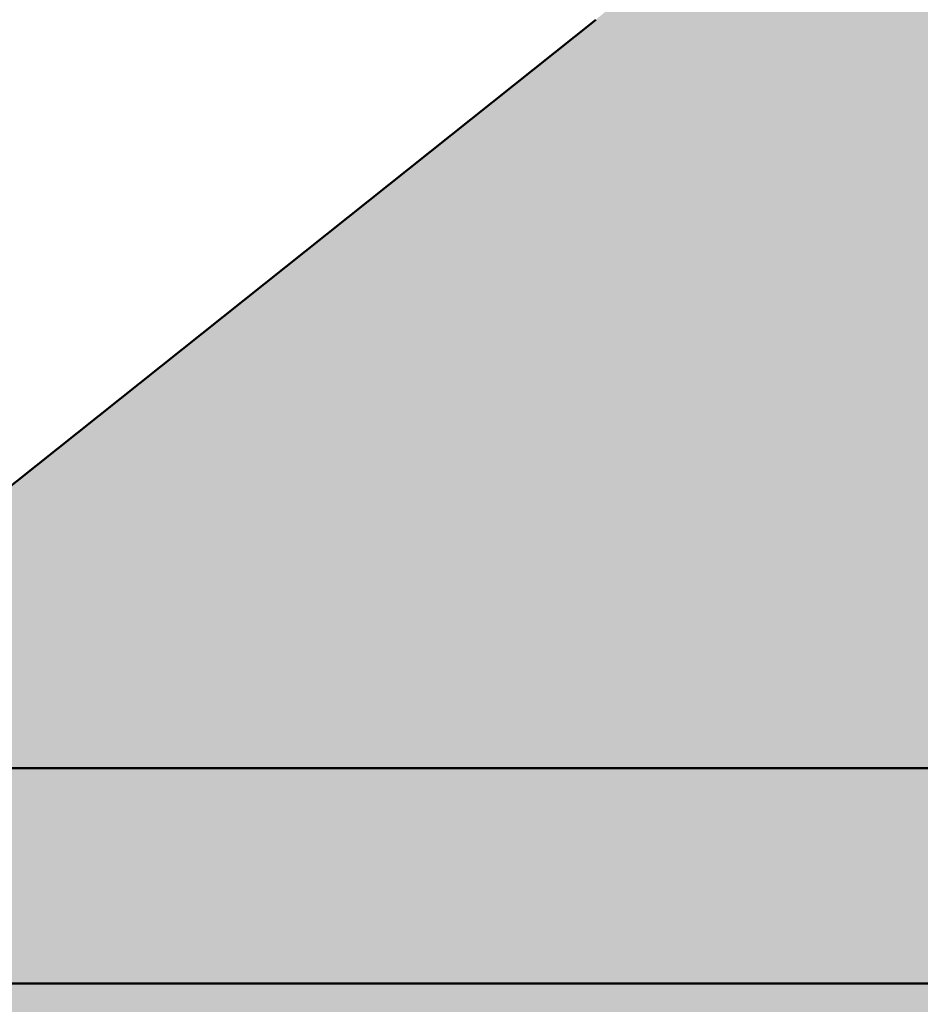
# Model space of a CAD drawing. Units: millimetres. Extents: x 0 to 2267, y 0 to 1823.
# Tile 20 of 256: x 1548 to 1590, y 1116 to 1162. Entities that reach past the tile are written whole.
import ezdxf

# ---------------------------------------------------------------- set-up
doc = ezdxf.new("R2010")
doc.units = ezdxf.units.MM
doc.header["$MEASUREMENT"] = 0
doc.layers.add('M-HATC', color=252, linetype='Continuous', lineweight=18)
doc.layers.add('M-OUTL', color=7, linetype='Continuous', lineweight=50)

msp = doc.modelspace()

# ---------------------------------------------------------------- hatches: boundary and pattern name
at = {"layer": 'M-HATC'}
h = msp.add_hatch(color=256, dxfattribs=at)
h.dxf.hatch_style = 1
h.paths.add_polyline_path([(2065.771, 1618.062, 0.236068), (2055.771, 1638.062), (1381.087, 1638.062, 0.236068), (1371.087, 1618.062), (1371.087, 1603.062), (2055.771, 1603.062), (2065.771, 1603.062)])
h.paths.add_polyline_path([(2062.772, 1550.296), (2062.772, 1560.296), (1374.086, 1560.296), (1374.086, 1550.296), (1374.086, 1540.296), (1384.086, 1540.296), (1389.086, 1540.296), (2062.772, 1540.296)])
h.paths.add_polyline_path([(1930.929, 1282.766), (1505.929, 1282.766), (1587.628, 1235.597, 0.131652), (1600.128, 1232.247), (1836.73, 1232.247, 0.131652), (1849.23, 1235.597)])
h.paths.add_polyline_path([(1930.929, 1117.417), (1905.929, 1117.417), (1505.929, 1117.417), (1505.929, 1077.417), (1930.929, 1077.417)])
h = msp.add_hatch(color=256, dxfattribs=at)
h.dxf.hatch_style = 1
h.paths.add_polyline_path([(2055.771, 1603.062), (1381.087, 1603.062), (1381.087, 1598.062), (2055.771, 1598.062)])
h.paths.add_polyline_path([(2055.771, 1598.062), (1381.087, 1598.062), (1381.087, 1593.062), (2055.771, 1593.062)])
h.paths.add_polyline_path([(2051.307, 1536.761), (1385.55, 1536.761), (1385.55, 1526.761), (1387.55, 1526.761), (1388.537, 1525.053), (1385.332, 1521.233), (1385.332, 1521.223), (2050.254, 1522.749), (2048.321, 1525.053), (2049.307, 1526.761), (2051.307, 1526.761)])
edge = h.paths.add_edge_path()
edge.add_arc((1847.535, 1379.149), 135, 222.60306, 222.89085, ccw=False)
edge.add_line((1748.166, 1287.766), (1683.092, 1287.766))
edge.add_arc((1583.724, 1379.149), 135, 317.10915, 317.39694, ccw=False)
edge.add_arc((1678.969, 1290.671), 5, 222.8909, 317.1091, ccw=False)
edge.add_arc((1774.213, 1379.149), 135, 222.60306, 222.89085, ccw=False)
edge.add_line((1674.845, 1287.766), (1609.771, 1287.766))
edge.add_arc((1510.403, 1379.149), 135, 317.10915, 317.39694, ccw=False)
edge.add_arc((1605.647, 1290.671), 5, 222.8909, 317.1091, ccw=False)
edge.add_arc((1700.892, 1379.149), 135, 222.60306, 222.89085, ccw=False)
edge.add_line((1601.524, 1287.766), (1536.45, 1287.766))
edge.add_arc((1437.081, 1379.149), 135, 317.10915, 317.39694, ccw=False)
edge.add_arc((1532.326, 1290.671), 5, 222.8909, 317.1091, ccw=False)
edge.add_arc((1627.571, 1379.149), 135, 222.60306, 222.89085, ccw=False)
edge.add_line((1528.203, 1287.766), (1505.929, 1287.766))
edge.add_spline(control_points=[(1505.929, 1287.766), (1504.262, 1287.766), (1504.262, 1282.766), (1505.929, 1282.766)], knot_values=[0, 0, 0, 0, 5, 5, 5, 5], degree=3, periodic=0)
edge.add_line((1505.929, 1282.766), (1930.929, 1282.766))
edge.add_spline(control_points=[(1930.929, 1282.766), (1932.596, 1282.766), (1932.596, 1287.766), (1930.929, 1287.766)], knot_values=[0, 0, 0, 0, 5, 5, 5, 5], degree=3, periodic=0)
edge.add_line((1930.929, 1287.766), (1903.056, 1287.766))
edge.add_arc((1803.688, 1379.149), 135, 317.10915, 317.39694, ccw=False)
edge.add_arc((1898.932, 1290.671), 5, 222.8909, 317.1091, ccw=False)
edge.add_arc((1994.177, 1379.149), 135, 222.60306, 222.89085, ccw=False)
edge.add_line((1894.809, 1287.766), (1829.735, 1287.766))
edge.add_arc((1730.366, 1379.149), 135, 317.10915, 317.39694, ccw=False)
edge.add_arc((1825.611, 1290.671), 5, 222.8909, 317.1091, ccw=False)
edge.add_arc((1920.856, 1379.149), 135, 222.60306, 222.89085, ccw=False)
edge.add_line((1821.487, 1287.766), (1756.413, 1287.766))
edge.add_arc((1657.045, 1379.149), 135, 317.10915, 317.39694, ccw=False)
edge.add_arc((1752.29, 1290.671), 5, 222.8909, 317.1091, ccw=False)
edge = h.paths.add_edge_path()
edge.add_spline(control_points=[(1843.429, 1227.247), (1845.096, 1227.247), (1845.096, 1232.247), (1843.429, 1232.247)], knot_values=[0, 0, 0, 0, 5, 5, 5, 5], degree=3, periodic=0)
edge.add_line((1843.429, 1232.247), (1593.429, 1232.247))
edge.add_spline(control_points=[(1593.429, 1232.247), (1591.762, 1232.247), (1591.762, 1227.247), (1593.429, 1227.247)], knot_values=[0, 0, 0, 0, 5, 5, 5, 5], degree=3, periodic=0)
edge.add_line((1593.429, 1227.247), (1843.429, 1227.247))
h.paths.add_polyline_path([(1905.929, 1127.417), (1530.929, 1127.417, 0.414214), (1520.929, 1117.417), (1530.929, 1117.417), (1915.929, 1117.417, 0.414214)])
edge = h.paths.add_edge_path()
edge.add_arc((1397.086, 1498.408), 12.73, 90.7821, 190.8787, ccw=False)
edge.add_line((1396.912, 1511.136), (1428.01, 1511.349))
edge.add_line((1428.01, 1511.349), (1433.01, 1511.349))
edge.add_line((1433.01, 1511.349), (1434.439, 1511.349))
edge.add_arc((1419.474, 1498.08), 20, 41.561, 74.0821)
edge.add_line((1424.959, 1517.314), (1399.935, 1517.256))
edge.add_spline(control_points=[(1399.931, 1517.256), (1399.884, 1517.213), (1399.833, 1517.169), (1399.777, 1517.124)], knot_values=[11.567499, 11.567499, 11.567499, 11.567499, 11.814249, 11.814249, 11.814249, 11.814249], degree=3, periodic=0)
edge.add_spline(control_points=[(1399.633, 1517.01), (1399.583, 1516.972), (1399.531, 1516.934), (1399.476, 1516.895)], knot_values=[11.167718, 11.167718, 11.167718, 11.167718, 11.365188, 11.365188, 11.365188, 11.365188], degree=3, periodic=0)
edge.add_spline(control_points=[(1399.34, 1516.8), (1399.151, 1516.672), (1398.938, 1516.538), (1398.704, 1516.399)], knot_values=[10.376405, 10.376405, 10.376405, 10.376405, 11.00994, 11.00994, 11.00994, 11.00994], degree=3, periodic=0)
edge.add_spline(control_points=[(1398.657, 1516.372), (1398.579, 1516.326), (1398.498, 1516.28), (1398.415, 1516.233)], knot_values=[10.125175, 10.125175, 10.125175, 10.125175, 10.334406, 10.334406, 10.334406, 10.334406], degree=3, periodic=0)
edge.add_spline(control_points=[(1398.264, 1516.149), (1398.196, 1516.111), (1398.126, 1516.073), (1398.055, 1516.035)], knot_values=[9.832246, 9.832246, 9.832246, 9.832246, 9.999658, 9.999658, 9.999658, 9.999658], degree=3, periodic=0)
edge.add_spline(control_points=[(1397.999, 1516.005), (1397.731, 1515.862), (1397.446, 1515.717), (1397.147, 1515.571)], knot_values=[9.161808, 9.161808, 9.161808, 9.161808, 9.787769, 9.787769, 9.787769, 9.787769], degree=3, periodic=0)
edge.add_spline(control_points=[(1397.147, 1515.571), (1396.842, 1515.423), (1396.522, 1515.274), (1396.191, 1515.126)], knot_values=[8.524455, 8.524455, 8.524455, 8.524455, 9.161808, 9.161808, 9.161808, 9.161808], degree=3, periodic=0)
edge.add_spline(control_points=[(1396.078, 1515.076), (1395.985, 1515.035), (1395.892, 1514.994), (1395.798, 1514.953)], knot_values=[8.275193, 8.275193, 8.275193, 8.275193, 8.451726, 8.451726, 8.451726, 8.451726], degree=3, periodic=0)
edge.add_spline(control_points=[(1395.602, 1514.869), (1395.5, 1514.826), (1395.397, 1514.782), (1395.293, 1514.739)], knot_values=[7.962917, 7.962917, 7.962917, 7.962917, 8.152764, 8.152764, 8.152764, 8.152764], degree=3, periodic=0)
edge.add_spline(control_points=[(1395.212, 1514.706), (1394.828, 1514.547), (1394.435, 1514.393), (1394.036, 1514.244)], knot_values=[7.21254, 7.21254, 7.21254, 7.21254, 7.913148, 7.913148, 7.913148, 7.913148], degree=3, periodic=0)
edge.add_spline(control_points=[(1394.036, 1514.244), (1393.708, 1514.121), (1393.375, 1514.003), (1393.043, 1513.889)], knot_values=[6.633733, 6.633733, 6.633733, 6.633733, 7.21254, 7.21254, 7.21254, 7.21254], degree=3, periodic=0)
edge.add_spline(control_points=[(1392.821, 1513.815), (1392.72, 1513.781), (1392.618, 1513.748), (1392.517, 1513.715)], knot_values=[6.328796, 6.328796, 6.328796, 6.328796, 6.505493, 6.505493, 6.505493, 6.505493], degree=3, periodic=0)
edge.add_spline(control_points=[(1392.517, 1513.715), (1392.319, 1513.652), (1392.121, 1513.59), (1391.924, 1513.531)], knot_values=[5.984605, 5.984605, 5.984605, 5.984605, 6.328796, 6.328796, 6.328796, 6.328796], degree=3, periodic=0)
edge.add_spline(control_points=[(1391.792, 1513.491), (1391.312, 1513.35), (1390.838, 1513.224), (1390.378, 1513.117)], knot_values=[5.066697, 5.066697, 5.066697, 5.066697, 5.907055, 5.907055, 5.907055, 5.907055], degree=3, periodic=0)
edge.add_spline(control_points=[(1390.378, 1513.117), (1390.18, 1513.071), (1389.984, 1513.028), (1389.791, 1512.99)], knot_values=[4.70367, 4.70367, 4.70367, 4.70367, 5.066695, 5.066695, 5.066695, 5.066695], degree=3, periodic=0)
edge.add_spline(control_points=[(1389.422, 1512.92), (1389.246, 1512.889), (1389.073, 1512.862), (1388.904, 1512.838)], knot_values=[4.130571, 4.130571, 4.130571, 4.130571, 4.469816, 4.469816, 4.469816, 4.469816], degree=3, periodic=0)
edge.add_spline(control_points=[(1388.904, 1512.838), (1388.591, 1512.795), (1388.291, 1512.764), (1388.007, 1512.749)], knot_values=[3.504031, 3.504031, 3.504031, 3.504031, 4.130571, 4.130571, 4.130571, 4.130571], degree=3, periodic=0)
edge.add_spline(control_points=[(1387.936, 1512.746), (1387.854, 1512.742), (1387.773, 1512.74), (1387.694, 1512.739)], knot_values=[3.268866, 3.268866, 3.268866, 3.268866, 3.451164, 3.451164, 3.451164, 3.451164], degree=3, periodic=0)
edge.add_spline(control_points=[(1387.335, 1512.744), (1387.208, 1512.75), (1387.085, 1512.76), (1386.967, 1512.774)], knot_values=[2.670686, 2.670686, 2.670686, 2.670686, 2.984, 2.984, 2.984, 2.984], degree=3, periodic=0)
edge.add_spline(control_points=[(1386.833, 1512.792), (1386.821, 1512.794), (1386.809, 1512.796), (1386.797, 1512.798)], knot_values=[2.516981, 2.516981, 2.516981, 2.516981, 2.549528, 2.549528, 2.549528, 2.549528], degree=3, periodic=0)
edge.add_spline(control_points=[(1386.453, 1512.873), (1386.426, 1512.881), (1386.399, 1512.889), (1386.373, 1512.897)], knot_values=[2.095869, 2.095869, 2.095869, 2.095869, 2.17941, 2.17941, 2.17941, 2.17941], degree=3, periodic=0)
edge.add_spline(control_points=[(1386.069, 1513.019), (1386.063, 1513.022), (1386.058, 1513.025), (1386.052, 1513.028)], knot_values=[1.72453, 1.72453, 1.72453, 1.72453, 1.745933, 1.745933, 1.745933, 1.745933], degree=3, periodic=0)
edge.add_arc((1399.474, 1498.08), 20, 131.8243, 180)
edge.add_arc((1630.334, 1505.548), 250.971, 181.70518, 236.42798)
edge.add_arc((1605.34, 1483.304), 218.782, 238.66083, 243.34961)
edge.add_arc((1647.091, 1510.359), 262.899, 183.12984, 237.85344, ccw=False)
h.paths.add_polyline_path([(1406.537, 1391.964, 0.149382), (1491.551, 1296.442, -0.129517)], flags=17)
edge = h.paths.add_edge_path()
edge.add_arc((2037.384, 1498.08), 20, 0, 48.2659)
edge.add_spline(control_points=[(2050.697, 1513.005), (2050.651, 1512.985), (2050.603, 1512.966), (2050.554, 1512.948)], knot_values=[1.835652, 1.835652, 1.835652, 1.835652, 2.000781, 2.000781, 2.000781, 2.000781], degree=3, periodic=0)
edge.add_spline(control_points=[(2050.462, 1512.917), (2050.479, 1512.922), (2050.496, 1512.928), (2050.513, 1512.934)], knot_values=[2.045477, 2.045477, 2.045477, 2.045477, 2.101389, 2.101389, 2.101389, 2.101389], degree=3, periodic=0)
edge.add_spline(control_points=[(2050.129, 1512.834), (2050.198, 1512.847), (2050.266, 1512.862), (2050.331, 1512.879)], knot_values=[2.237629, 2.237629, 2.237629, 2.237629, 2.435841, 2.435841, 2.435841, 2.435841], degree=3, periodic=0)
edge.add_spline(control_points=[(2050.095, 1512.828), (2050.106, 1512.83), (2050.118, 1512.832), (2050.129, 1512.834)], knot_values=[2.435841, 2.435841, 2.435841, 2.435841, 2.468321, 2.468321, 2.468321, 2.468321], degree=3, periodic=0)
edge.add_spline(control_points=[(2049.784, 1512.785), (2049.855, 1512.792), (2049.924, 1512.801), (2049.992, 1512.811)], knot_values=[2.563852, 2.563852, 2.563852, 2.563852, 2.748541, 2.748541, 2.748541, 2.748541], degree=3, periodic=0)
edge.add_spline(control_points=[(2049.405, 1512.762), (2049.536, 1512.765), (2049.663, 1512.773), (2049.784, 1512.785)], knot_values=[2.748541, 2.748541, 2.748541, 2.748541, 3.064882, 3.064882, 3.064882, 3.064882], degree=3, periodic=0)
edge.add_spline(control_points=[(2049.17, 1512.76), (2049.234, 1512.759), (2049.297, 1512.759), (2049.358, 1512.761)], knot_values=[3.102309, 3.102309, 3.102309, 3.102309, 3.2503, 3.2503, 3.2503, 3.2503], degree=3, periodic=0)
edge.add_spline(control_points=[(2048.857, 1512.769), (2048.964, 1512.764), (2049.068, 1512.761), (2049.17, 1512.76)], knot_values=[3.2503, 3.2503, 3.2503, 3.2503, 3.486069, 3.486069, 3.486069, 3.486069], degree=3, periodic=0)
edge.add_spline(control_points=[(2048.692, 1512.779), (2048.373, 1512.801), (2048.035, 1512.841), (2047.682, 1512.897)], knot_values=[3.606429, 3.606429, 3.606429, 3.606429, 4.2989, 4.2989, 4.2989, 4.2989], degree=3, periodic=0)
edge.add_spline(control_points=[(2047.682, 1512.897), (2047.546, 1512.919), (2047.408, 1512.942), (2047.268, 1512.969)], knot_values=[4.2989, 4.2989, 4.2989, 4.2989, 4.565769, 4.565769, 4.565769, 4.565769], degree=3, periodic=0)
edge.add_spline(control_points=[(2047.268, 1512.969), (2047.145, 1512.991), (2047.021, 1513.016), (2046.895, 1513.042)], knot_values=[4.565769, 4.565769, 4.565769, 4.565769, 4.799971, 4.799971, 4.799971, 4.799971], degree=3, periodic=0)
edge.add_spline(control_points=[(2046.895, 1513.042), (2046.529, 1513.119), (2046.151, 1513.209), (2045.768, 1513.311)], knot_values=[4.799971, 4.799971, 4.799971, 4.799971, 5.483718, 5.483718, 5.483718, 5.483718], degree=3, periodic=0)
edge.add_spline(control_points=[(2045.768, 1513.311), (2045.372, 1513.415), (2044.97, 1513.532), (2044.566, 1513.659)], knot_values=[5.483718, 5.483718, 5.483718, 5.483718, 6.187866, 6.187866, 6.187866, 6.187866], degree=3, periodic=0)
edge.add_spline(control_points=[(2044.566, 1513.659), (2044.415, 1513.706), (2044.263, 1513.755), (2044.112, 1513.805)], knot_values=[6.187866, 6.187866, 6.187866, 6.187866, 6.451551, 6.451551, 6.451551, 6.451551], degree=3, periodic=0)
edge.add_spline(control_points=[(2044.112, 1513.805), (2043.997, 1513.843), (2043.882, 1513.881), (2043.767, 1513.92)], knot_values=[6.451551, 6.451551, 6.451551, 6.451551, 6.651434, 6.651434, 6.651434, 6.651434], degree=3, periodic=0)
edge.add_spline(control_points=[(2043.767, 1513.92), (2043.372, 1514.055), (2042.977, 1514.198), (2042.589, 1514.346)], knot_values=[6.651434, 6.651434, 6.651434, 6.651434, 7.338879, 7.338879, 7.338879, 7.338879], degree=3, periodic=0)
edge.add_spline(control_points=[(2042.589, 1514.346), (2042.164, 1514.507), (2041.746, 1514.675), (2041.341, 1514.846)], knot_values=[7.338879, 7.338879, 7.338879, 7.338879, 8.089209, 8.089209, 8.089209, 8.089209], degree=3, periodic=0)
edge.add_spline(control_points=[(2041.341, 1514.846), (2041.103, 1514.946), (2040.869, 1515.048), (2040.64, 1515.15)], knot_values=[8.089209, 8.089209, 8.089209, 8.089209, 8.529587, 8.529587, 8.529587, 8.529587], degree=3, periodic=0)
edge.add_spline(control_points=[(2040.51, 1515.209), (2040.082, 1515.402), (2039.675, 1515.597), (2039.295, 1515.789)], knot_values=[8.613818, 8.613818, 8.613818, 8.613818, 9.44571, 9.44571, 9.44571, 9.44571], degree=3, periodic=0)
edge.add_spline(control_points=[(2039.295, 1515.789), (2039.062, 1515.907), (2038.839, 1516.025), (2038.629, 1516.14)], knot_values=[9.44571, 9.44571, 9.44571, 9.44571, 9.956404, 9.956404, 9.956404, 9.956404], degree=3, periodic=0)
edge.add_spline(control_points=[(2038.629, 1516.14), (2038.519, 1516.2), (2038.412, 1516.26), (2038.309, 1516.319)], knot_values=[9.956404, 9.956404, 9.956404, 9.956404, 10.223542, 10.223542, 10.223542, 10.223542], degree=3, periodic=0)
edge.add_spline(control_points=[(2038.309, 1516.319), (2038.214, 1516.374), (2038.122, 1516.428), (2038.033, 1516.481)], knot_values=[10.223542, 10.223542, 10.223542, 10.223542, 10.47051, 10.47051, 10.47051, 10.47051], degree=3, periodic=0)
edge.add_spline(control_points=[(2038.033, 1516.481), (2037.786, 1516.63), (2037.564, 1516.773), (2037.372, 1516.909)], knot_values=[10.47051, 10.47051, 10.47051, 10.47051, 11.15767, 11.15767, 11.15767, 11.15767], degree=3, periodic=0)
edge.add_spline(control_points=[(2037.372, 1516.909), (2037.279, 1516.975), (2037.193, 1517.04), (2037.114, 1517.102)], knot_values=[11.15767, 11.15767, 11.15767, 11.15767, 11.49227, 11.49227, 11.49227, 11.49227], degree=3, periodic=0)
edge.add_spline(control_points=[(2036.856, 1517.326), (2036.915, 1517.269), (2036.981, 1517.21), (2037.056, 1517.149)], knot_values=[11.577341, 11.577341, 11.577341, 11.577341, 11.91035, 11.91035, 11.91035, 11.91035], degree=3, periodic=0)
edge.add_spline(control_points=[(2036.807, 1517.375), (2036.823, 1517.359), (2036.839, 1517.342), (2036.856, 1517.326)], knot_values=[11.91035, 11.91035, 11.91035, 11.91035, 12.007402, 12.007402, 12.007402, 12.007402], degree=3, periodic=0)
edge.add_spline(control_points=[(2036.702, 1517.494), (2036.71, 1517.483), (2036.72, 1517.472), (2036.729, 1517.461)], knot_values=[12.184155, 12.184155, 12.184155, 12.184155, 12.255409, 12.255409, 12.255409, 12.255409], degree=3, periodic=0)
edge.add_spline(control_points=[(2036.616, 1517.621), (2036.62, 1517.613), (2036.624, 1517.606), (2036.629, 1517.598)], knot_values=[12.487913, 12.487913, 12.487913, 12.487913, 12.541035, 12.541035, 12.541035, 12.541035], degree=3, periodic=0)
edge.add_spline(control_points=[(2036.563, 1517.786), (2036.564, 1517.779), (2036.564, 1517.773), (2036.565, 1517.766)], knot_values=[12.911761, 12.911761, 12.911761, 12.911761, 12.968286, 12.968286, 12.968286, 12.968286], degree=3, periodic=0)
edge.add_spline(control_points=[(2036.617, 1517.93), (2036.612, 1517.926), (2036.609, 1517.921), (2036.605, 1517.916)], knot_values=[13.382527, 13.382527, 13.382527, 13.382527, 13.433791, 13.433791, 13.433791, 13.433791], degree=3, periodic=0)
edge.add_spline(control_points=[(2036.749, 1518.017), (2036.736, 1518.012), (2036.724, 1518.006), (2036.712, 1518)], knot_values=[13.726299, 13.726299, 13.726299, 13.726299, 13.809928, 13.809928, 13.809928, 13.809928], degree=3, periodic=0)
edge.add_spline(control_points=[(2036.86, 1518.053), (2036.839, 1518.047), (2036.818, 1518.042), (2036.799, 1518.035)], knot_values=[13.910887, 13.910887, 13.910887, 13.910887, 14.02153, 14.02153, 14.02153, 14.02153], degree=3, periodic=0)
edge.add_line((2036.964, 1518.08), (2032.384, 1518.08))
edge.add_line((2032.384, 1518.08), (2027.384, 1518.08))
edge.add_line((2027.384, 1518.08), (2022.384, 1518.08))
edge.add_line((2022.384, 1518.08), (2017.384, 1518.08))
edge.add_arc((2017.384, 1498.08), 20, 90, 138.439)
edge.add_line((2002.419, 1511.349), (2003.848, 1511.349))
edge.add_line((2003.848, 1511.349), (2008.848, 1511.349))
edge.add_line((2008.848, 1511.349), (2039.772, 1511.138))
edge.add_arc((2039.772, 1498.408), 12.73, -10.8787, 90, ccw=False)
edge.add_arc((1789.767, 1510.359), 262.899, 302.14656, 356.87016, ccw=False)
edge.add_arc((1831.518, 1483.304), 218.782, 296.65039, 301.33917)
edge.add_arc((1806.524, 1505.548), 250.971, 303.57202, 358.29482)
h.paths.add_polyline_path([(2030.321, 1391.964, -0.129517), (1945.307, 1296.442, 0.149382)], flags=17)
edge = h.paths.add_edge_path()
edge.add_spline(control_points=[(2037.246, 1518.082), (2037.29, 1518.081), (2037.336, 1518.08), (2037.384, 1518.08)], knot_values=[0.000012, 0.000012, 0.000012, 0.000012, 0.144754, 0.144754, 0.144754, 0.144754], degree=3, periodic=0)
edge.add_line((2037.336, 1518.08), (2037.01, 1518.08))
edge.add_spline(control_points=[(2037.01, 1518.08), (2036.982, 1518.077), (2036.956, 1518.073), (2036.931, 1518.068)], knot_values=[14.13465, 14.13465, 14.13465, 14.13465, 14.247197, 14.247197, 14.247197, 14.247197], degree=3, periodic=0)
edge.add_spline(control_points=[(2036.931, 1518.068), (2036.928, 1518.067), (2036.924, 1518.067), (2036.921, 1518.066)], knot_values=[14.118315, 14.118315, 14.118315, 14.118315, 14.13465, 14.13465, 14.13465, 14.13465], degree=3, periodic=0)
edge.add_spline(control_points=[(2036.921, 1518.066), (2036.912, 1518.064), (2036.903, 1518.063), (2036.895, 1518.061)], knot_values=[14.078086, 14.078086, 14.078086, 14.078086, 14.118315, 14.118315, 14.118315, 14.118315], degree=3, periodic=0)
edge.add_spline(control_points=[(2036.895, 1518.061), (2036.883, 1518.058), (2036.872, 1518.056), (2036.86, 1518.053)], knot_values=[14.02153, 14.02153, 14.02153, 14.02153, 14.078086, 14.078086, 14.078086, 14.078086], degree=3, periodic=0)
edge.add_spline(control_points=[(2036.86, 1518.053), (2036.839, 1518.047), (2036.818, 1518.042), (2036.799, 1518.035)], knot_values=[13.910887, 13.910887, 13.910887, 13.910887, 14.02153, 14.02153, 14.02153, 14.02153], degree=3, periodic=0)
edge.add_spline(control_points=[(2036.799, 1518.035), (2036.798, 1518.035), (2036.797, 1518.035), (2036.797, 1518.035)], knot_values=[13.906906, 13.906906, 13.906906, 13.906906, 13.910887, 13.910887, 13.910887, 13.910887], degree=3, periodic=0)
edge.add_spline(control_points=[(2036.797, 1518.035), (2036.788, 1518.032), (2036.78, 1518.029), (2036.772, 1518.026)], knot_values=[13.857826, 13.857826, 13.857826, 13.857826, 13.906906, 13.906906, 13.906906, 13.906906], degree=3, periodic=0)
edge.add_spline(control_points=[(2036.772, 1518.026), (2036.764, 1518.023), (2036.756, 1518.02), (2036.749, 1518.017)], knot_values=[13.809928, 13.809928, 13.809928, 13.809928, 13.857826, 13.857826, 13.857826, 13.857826], degree=3, periodic=0)
edge.add_spline(control_points=[(2036.749, 1518.017), (2036.736, 1518.012), (2036.724, 1518.006), (2036.712, 1518)], knot_values=[13.726299, 13.726299, 13.726299, 13.726299, 13.809928, 13.809928, 13.809928, 13.809928], degree=3, periodic=0)
edge.add_spline(control_points=[(2036.712, 1518), (2036.712, 1518), (2036.712, 1518), (2036.711, 1518)], knot_values=[13.723993, 13.723993, 13.723993, 13.723993, 13.726299, 13.726299, 13.726299, 13.726299], degree=3, periodic=0)
edge.add_spline(control_points=[(2036.711, 1518), (2036.706, 1517.997), (2036.701, 1517.994), (2036.696, 1517.992)], knot_values=[13.686536, 13.686536, 13.686536, 13.686536, 13.723993, 13.723993, 13.723993, 13.723993], degree=3, periodic=0)
edge.add_spline(control_points=[(2036.696, 1517.992), (2036.692, 1517.989), (2036.687, 1517.987), (2036.683, 1517.984)], knot_values=[13.651251, 13.651251, 13.651251, 13.651251, 13.686536, 13.686536, 13.686536, 13.686536], degree=3, periodic=0)
edge.add_spline(control_points=[(2036.683, 1517.984), (2036.676, 1517.98), (2036.67, 1517.976), (2036.664, 1517.971)], knot_values=[13.596804, 13.596804, 13.596804, 13.596804, 13.651251, 13.651251, 13.651251, 13.651251], degree=3, periodic=0)
edge.add_spline(control_points=[(2036.664, 1517.971), (2036.664, 1517.971), (2036.663, 1517.971), (2036.663, 1517.971)], knot_values=[13.593956, 13.593956, 13.593956, 13.593956, 13.596804, 13.596804, 13.596804, 13.596804], degree=3, periodic=0)
edge.add_spline(control_points=[(2036.663, 1517.971), (2036.66, 1517.969), (2036.658, 1517.967), (2036.655, 1517.965)], knot_values=[13.570322, 13.570322, 13.570322, 13.570322, 13.593956, 13.593956, 13.593956, 13.593956], degree=3, periodic=0)
edge.add_spline(control_points=[(2036.655, 1517.965), (2036.653, 1517.963), (2036.65, 1517.961), (2036.647, 1517.959)], knot_values=[13.545477, 13.545477, 13.545477, 13.545477, 13.570322, 13.570322, 13.570322, 13.570322], degree=3, periodic=0)
edge.add_spline(control_points=[(2036.647, 1517.959), (2036.647, 1517.959), (2036.647, 1517.959), (2036.647, 1517.959)], knot_values=[13.543931, 13.543931, 13.543931, 13.543931, 13.545477, 13.545477, 13.545477, 13.545477], degree=3, periodic=0)
edge.add_spline(control_points=[(2036.647, 1517.959), (2036.641, 1517.954), (2036.636, 1517.949), (2036.631, 1517.945)], knot_values=[13.488237, 13.488237, 13.488237, 13.488237, 13.543931, 13.543931, 13.543931, 13.543931], degree=3, periodic=0)
edge.add_spline(control_points=[(2036.631, 1517.945), (2036.628, 1517.942), (2036.626, 1517.94), (2036.623, 1517.937)], knot_values=[13.460307, 13.460307, 13.460307, 13.460307, 13.488237, 13.488237, 13.488237, 13.488237], degree=3, periodic=0)
edge.add_spline(control_points=[(2036.623, 1517.937), (2036.622, 1517.936), (2036.62, 1517.934), (2036.618, 1517.932)], knot_values=[13.439712, 13.439712, 13.439712, 13.439712, 13.460307, 13.460307, 13.460307, 13.460307], degree=3, periodic=0)
edge.add_spline(control_points=[(2036.618, 1517.932), (2036.618, 1517.931), (2036.617, 1517.931), (2036.617, 1517.93)], knot_values=[13.433791, 13.433791, 13.433791, 13.433791, 13.439712, 13.439712, 13.439712, 13.439712], degree=3, periodic=0)
edge.add_spline(control_points=[(2036.617, 1517.93), (2036.612, 1517.926), (2036.609, 1517.921), (2036.605, 1517.916)], knot_values=[13.382527, 13.382527, 13.382527, 13.382527, 13.433791, 13.433791, 13.433791, 13.433791], degree=3, periodic=0)
edge.add_spline(control_points=[(2036.605, 1517.916), (2036.603, 1517.913), (2036.6, 1517.91), (2036.598, 1517.907)], knot_values=[13.350017, 13.350017, 13.350017, 13.350017, 13.382527, 13.382527, 13.382527, 13.382527], degree=3, periodic=0)
edge.add_spline(control_points=[(2036.598, 1517.907), (2036.597, 1517.906), (2036.596, 1517.904), (2036.595, 1517.903)], knot_values=[13.333922, 13.333922, 13.333922, 13.333922, 13.350017, 13.350017, 13.350017, 13.350017], degree=3, periodic=0)
edge.add_spline(control_points=[(2036.595, 1517.903), (2036.595, 1517.902), (2036.594, 1517.901), (2036.593, 1517.9)], knot_values=[13.323828, 13.323828, 13.323828, 13.323828, 13.333922, 13.333922, 13.333922, 13.333922], degree=3, periodic=0)
edge.add_spline(control_points=[(2036.593, 1517.9), (2036.59, 1517.895), (2036.588, 1517.891), (2036.585, 1517.886)], knot_values=[13.277545, 13.277545, 13.277545, 13.277545, 13.323828, 13.323828, 13.323828, 13.323828], degree=3, periodic=0)
edge.add_spline(control_points=[(2036.585, 1517.886), (2036.584, 1517.883), (2036.582, 1517.879), (2036.58, 1517.875)], knot_values=[13.240119, 13.240119, 13.240119, 13.240119, 13.277545, 13.277545, 13.277545, 13.277545], degree=3, periodic=0)
edge.add_spline(control_points=[(2036.58, 1517.875), (2036.58, 1517.874), (2036.579, 1517.873), (2036.578, 1517.872)], knot_values=[13.228211, 13.228211, 13.228211, 13.228211, 13.240119, 13.240119, 13.240119, 13.240119], degree=3, periodic=0)
edge.add_spline(control_points=[(2036.578, 1517.872), (2036.578, 1517.87), (2036.577, 1517.869), (2036.577, 1517.868)], knot_values=[13.215717, 13.215717, 13.215717, 13.215717, 13.228211, 13.228211, 13.228211, 13.228211], degree=3, periodic=0)
edge.add_spline(control_points=[(2036.577, 1517.868), (2036.575, 1517.864), (2036.574, 1517.86), (2036.573, 1517.857)], knot_values=[13.179847, 13.179847, 13.179847, 13.179847, 13.215717, 13.215717, 13.215717, 13.215717], degree=3, periodic=0)
edge.add_spline(control_points=[(2036.573, 1517.857), (2036.571, 1517.851), (2036.57, 1517.846), (2036.569, 1517.841)], knot_values=[13.132017, 13.132017, 13.132017, 13.132017, 13.179847, 13.179847, 13.179847, 13.179847], degree=3, periodic=0)
edge.add_spline(control_points=[(2036.569, 1517.841), (2036.568, 1517.84), (2036.568, 1517.839), (2036.568, 1517.838)], knot_values=[13.122482, 13.122482, 13.122482, 13.122482, 13.132017, 13.132017, 13.132017, 13.132017], degree=3, periodic=0)
edge.add_spline(control_points=[(2036.568, 1517.838), (2036.568, 1517.836), (2036.567, 1517.835), (2036.567, 1517.833)], knot_values=[13.105592, 13.105592, 13.105592, 13.105592, 13.122482, 13.122482, 13.122482, 13.122482], degree=3, periodic=0)
edge.add_spline(control_points=[(2036.567, 1517.833), (2036.566, 1517.829), (2036.566, 1517.826), (2036.565, 1517.822)], knot_values=[13.074063, 13.074063, 13.074063, 13.074063, 13.105592, 13.105592, 13.105592, 13.105592], degree=3, periodic=0)
edge.add_spline(control_points=[(2036.565, 1517.822), (2036.565, 1517.822), (2036.565, 1517.822), (2036.565, 1517.822)], knot_values=[13.074043, 13.074043, 13.074043, 13.074043, 13.074063, 13.074063, 13.074063, 13.074063], degree=3, periodic=0)
edge.add_spline(control_points=[(2036.565, 1517.822), (2036.564, 1517.816), (2036.564, 1517.811), (2036.564, 1517.805)], knot_values=[13.021884, 13.021884, 13.021884, 13.021884, 13.074043, 13.074043, 13.074043, 13.074043], degree=3, periodic=0)
edge.add_spline(control_points=[(2036.564, 1517.805), (2036.564, 1517.804), (2036.564, 1517.803), (2036.564, 1517.803)], knot_values=[13.01674, 13.01674, 13.01674, 13.01674, 13.021884, 13.021884, 13.021884, 13.021884], degree=3, periodic=0)
edge.add_spline(control_points=[(2036.564, 1517.803), (2036.563, 1517.801), (2036.563, 1517.798), (2036.563, 1517.796)], knot_values=[12.996438, 12.996438, 12.996438, 12.996438, 13.01674, 13.01674, 13.01674, 13.01674], degree=3, periodic=0)
edge.add_spline(control_points=[(2036.563, 1517.796), (2036.563, 1517.793), (2036.563, 1517.789), (2036.563, 1517.786)], knot_values=[12.968286, 12.968286, 12.968286, 12.968286, 12.996438, 12.996438, 12.996438, 12.996438], degree=3, periodic=0)
edge.add_spline(control_points=[(2036.563, 1517.786), (2036.564, 1517.779), (2036.564, 1517.773), (2036.565, 1517.766)], knot_values=[12.911761, 12.911761, 12.911761, 12.911761, 12.968286, 12.968286, 12.968286, 12.968286], degree=3, periodic=0)
edge.add_spline(control_points=[(2036.565, 1517.766), (2036.565, 1517.766), (2036.565, 1517.766), (2036.565, 1517.766)], knot_values=[12.911017, 12.911017, 12.911017, 12.911017, 12.911761, 12.911761, 12.911761, 12.911761], degree=3, periodic=0)
edge.add_spline(control_points=[(2036.565, 1517.766), (2036.565, 1517.762), (2036.566, 1517.759), (2036.566, 1517.756)], knot_values=[12.88528, 12.88528, 12.88528, 12.88528, 12.911017, 12.911017, 12.911017, 12.911017], degree=3, periodic=0)
edge.add_spline(control_points=[(2036.566, 1517.756), (2036.567, 1517.753), (2036.567, 1517.751), (2036.568, 1517.748)], knot_values=[12.862519, 12.862519, 12.862519, 12.862519, 12.88528, 12.88528, 12.88528, 12.88528], degree=3, periodic=0)
edge.add_spline(control_points=[(2036.568, 1517.748), (2036.568, 1517.747), (2036.568, 1517.747), (2036.568, 1517.746)], knot_values=[12.858885, 12.858885, 12.858885, 12.858885, 12.862519, 12.862519, 12.862519, 12.862519], degree=3, periodic=0)
edge.add_spline(control_points=[(2036.568, 1517.746), (2036.569, 1517.74), (2036.571, 1517.733), (2036.572, 1517.726)], knot_values=[12.8053, 12.8053, 12.8053, 12.8053, 12.858885, 12.858885, 12.858885, 12.858885], degree=3, periodic=0)
edge.add_spline(control_points=[(2036.572, 1517.726), (2036.573, 1517.723), (2036.574, 1517.719), (2036.576, 1517.715)], knot_values=[12.775176, 12.775176, 12.775176, 12.775176, 12.8053, 12.8053, 12.8053, 12.8053], degree=3, periodic=0)
edge.add_spline(control_points=[(2036.576, 1517.715), (2036.576, 1517.713), (2036.577, 1517.71), (2036.578, 1517.708)], knot_values=[12.756759, 12.756759, 12.756759, 12.756759, 12.775176, 12.775176, 12.775176, 12.775176], degree=3, periodic=0)
edge.add_spline(control_points=[(2036.578, 1517.708), (2036.578, 1517.707), (2036.578, 1517.706), (2036.579, 1517.705)], knot_values=[12.748742, 12.748742, 12.748742, 12.748742, 12.756759, 12.756759, 12.756759, 12.756759], degree=3, periodic=0)
edge.add_spline(control_points=[(2036.579, 1517.705), (2036.581, 1517.698), (2036.583, 1517.692), (2036.586, 1517.685)], knot_values=[12.69959, 12.69959, 12.69959, 12.69959, 12.748742, 12.748742, 12.748742, 12.748742], degree=3, periodic=0)
edge.add_spline(control_points=[(2036.586, 1517.685), (2036.588, 1517.68), (2036.59, 1517.675), (2036.592, 1517.669)], knot_values=[12.659038, 12.659038, 12.659038, 12.659038, 12.69959, 12.69959, 12.69959, 12.69959], degree=3, periodic=0)
edge.add_spline(control_points=[(2036.592, 1517.669), (2036.594, 1517.665), (2036.596, 1517.66), (2036.598, 1517.656)], knot_values=[12.626806, 12.626806, 12.626806, 12.626806, 12.659038, 12.659038, 12.659038, 12.659038], degree=3, periodic=0)
edge.add_spline(control_points=[(2036.598, 1517.656), (2036.598, 1517.655), (2036.599, 1517.654), (2036.599, 1517.653)], knot_values=[12.619394, 12.619394, 12.619394, 12.619394, 12.626806, 12.626806, 12.626806, 12.626806], degree=3, periodic=0)
edge.add_spline(control_points=[(2036.599, 1517.653), (2036.604, 1517.642), (2036.61, 1517.632), (2036.616, 1517.621)], knot_values=[12.541039, 12.541039, 12.541039, 12.541039, 12.619394, 12.619394, 12.619394, 12.619394], degree=3, periodic=0)
edge.add_spline(control_points=[(2036.616, 1517.621), (2036.616, 1517.621), (2036.616, 1517.621), (2036.616, 1517.621)], knot_values=[12.541035, 12.541035, 12.541035, 12.541035, 12.541039, 12.541039, 12.541039, 12.541039], degree=3, periodic=0)
edge.add_spline(control_points=[(2036.616, 1517.621), (2036.62, 1517.613), (2036.624, 1517.606), (2036.629, 1517.598)], knot_values=[12.487913, 12.487913, 12.487913, 12.487913, 12.541035, 12.541035, 12.541035, 12.541035], degree=3, periodic=0)
edge.add_spline(control_points=[(2036.629, 1517.598), (2036.633, 1517.592), (2036.637, 1517.585), (2036.641, 1517.579)], knot_values=[12.443982, 12.443982, 12.443982, 12.443982, 12.487913, 12.487913, 12.487913, 12.487913], degree=3, periodic=0)
edge.add_spline(control_points=[(2036.641, 1517.579), (2036.641, 1517.578), (2036.642, 1517.576), (2036.643, 1517.575)], knot_values=[12.434996, 12.434996, 12.434996, 12.434996, 12.443982, 12.443982, 12.443982, 12.443982], degree=3, periodic=0)
edge.add_spline(control_points=[(2036.643, 1517.575), (2036.653, 1517.56), (2036.664, 1517.544), (2036.676, 1517.528)], knot_values=[12.329647, 12.329647, 12.329647, 12.329647, 12.434996, 12.434996, 12.434996, 12.434996], degree=3, periodic=0)
edge.add_spline(control_points=[(2036.676, 1517.528), (2036.684, 1517.517), (2036.693, 1517.505), (2036.702, 1517.494)], knot_values=[12.255409, 12.255409, 12.255409, 12.255409, 12.329647, 12.329647, 12.329647, 12.329647], degree=3, periodic=0)
edge.add_spline(control_points=[(2036.702, 1517.494), (2036.71, 1517.483), (2036.72, 1517.472), (2036.729, 1517.461)], knot_values=[12.184155, 12.184155, 12.184155, 12.184155, 12.255409, 12.255409, 12.255409, 12.255409], degree=3, periodic=0)
edge.add_spline(control_points=[(2036.729, 1517.461), (2036.744, 1517.444), (2036.759, 1517.426), (2036.775, 1517.409)], knot_values=[12.075961, 12.075961, 12.075961, 12.075961, 12.184155, 12.184155, 12.184155, 12.184155], degree=3, periodic=0)
edge.add_spline(control_points=[(2036.775, 1517.409), (2036.776, 1517.407), (2036.777, 1517.406), (2036.778, 1517.405)], knot_values=[12.069502, 12.069502, 12.069502, 12.069502, 12.075961, 12.075961, 12.075961, 12.075961], degree=3, periodic=0)
edge.add_spline(control_points=[(2036.778, 1517.405), (2036.788, 1517.395), (2036.797, 1517.385), (2036.807, 1517.375)], knot_values=[12.007402, 12.007402, 12.007402, 12.007402, 12.069502, 12.069502, 12.069502, 12.069502], degree=3, periodic=0)
edge.add_spline(control_points=[(2036.807, 1517.375), (2036.823, 1517.359), (2036.839, 1517.342), (2036.856, 1517.326)], knot_values=[11.91035, 11.91035, 11.91035, 11.91035, 12.007402, 12.007402, 12.007402, 12.007402], degree=3, periodic=0)
edge.add_spline(control_points=[(2036.856, 1517.326), (2036.915, 1517.269), (2036.981, 1517.21), (2037.056, 1517.149)], knot_values=[11.577341, 11.577341, 11.577341, 11.577341, 11.91035, 11.91035, 11.91035, 11.91035], degree=3, periodic=0)
edge.add_spline(control_points=[(2037.056, 1517.149), (2037.075, 1517.134), (2037.094, 1517.118), (2037.114, 1517.102)], knot_values=[11.49227, 11.49227, 11.49227, 11.49227, 11.577341, 11.577341, 11.577341, 11.577341], degree=3, periodic=0)
edge.add_spline(control_points=[(2037.114, 1517.102), (2037.193, 1517.04), (2037.279, 1516.975), (2037.372, 1516.909)], knot_values=[11.15767, 11.15767, 11.15767, 11.15767, 11.49227, 11.49227, 11.49227, 11.49227], degree=3, periodic=0)
edge.add_spline(control_points=[(2037.372, 1516.909), (2037.564, 1516.773), (2037.786, 1516.63), (2038.033, 1516.481)], knot_values=[10.47051, 10.47051, 10.47051, 10.47051, 11.15767, 11.15767, 11.15767, 11.15767], degree=3, periodic=0)
edge.add_spline(control_points=[(2038.033, 1516.481), (2038.122, 1516.428), (2038.214, 1516.374), (2038.309, 1516.319)], knot_values=[10.223542, 10.223542, 10.223542, 10.223542, 10.47051, 10.47051, 10.47051, 10.47051], degree=3, periodic=0)
edge.add_spline(control_points=[(2038.309, 1516.319), (2038.412, 1516.26), (2038.519, 1516.2), (2038.629, 1516.14)], knot_values=[9.956404, 9.956404, 9.956404, 9.956404, 10.223542, 10.223542, 10.223542, 10.223542], degree=3, periodic=0)
edge.add_spline(control_points=[(2038.629, 1516.14), (2038.839, 1516.025), (2039.062, 1515.907), (2039.295, 1515.789)], knot_values=[9.44571, 9.44571, 9.44571, 9.44571, 9.956404, 9.956404, 9.956404, 9.956404], degree=3, periodic=0)
edge.add_spline(control_points=[(2039.295, 1515.789), (2039.675, 1515.597), (2040.082, 1515.402), (2040.51, 1515.209)], knot_values=[8.613818, 8.613818, 8.613818, 8.613818, 9.44571, 9.44571, 9.44571, 9.44571], degree=3, periodic=0)
edge.add_spline(control_points=[(2040.51, 1515.209), (2040.553, 1515.189), (2040.597, 1515.17), (2040.64, 1515.15)], knot_values=[8.529587, 8.529587, 8.529587, 8.529587, 8.613818, 8.613818, 8.613818, 8.613818], degree=3, periodic=0)
edge.add_spline(control_points=[(2040.64, 1515.15), (2040.869, 1515.048), (2041.103, 1514.946), (2041.341, 1514.846)], knot_values=[8.089209, 8.089209, 8.089209, 8.089209, 8.529587, 8.529587, 8.529587, 8.529587], degree=3, periodic=0)
edge.add_spline(control_points=[(2041.341, 1514.846), (2041.746, 1514.675), (2042.164, 1514.507), (2042.589, 1514.346)], knot_values=[7.338879, 7.338879, 7.338879, 7.338879, 8.089209, 8.089209, 8.089209, 8.089209], degree=3, periodic=0)
edge.add_spline(control_points=[(2042.589, 1514.346), (2042.977, 1514.198), (2043.372, 1514.055), (2043.767, 1513.92)], knot_values=[6.651434, 6.651434, 6.651434, 6.651434, 7.338879, 7.338879, 7.338879, 7.338879], degree=3, periodic=0)
edge.add_spline(control_points=[(2043.767, 1513.92), (2043.882, 1513.881), (2043.997, 1513.843), (2044.112, 1513.805)], knot_values=[6.451551, 6.451551, 6.451551, 6.451551, 6.651434, 6.651434, 6.651434, 6.651434], degree=3, periodic=0)
edge.add_spline(control_points=[(2044.112, 1513.805), (2044.263, 1513.755), (2044.415, 1513.706), (2044.566, 1513.659)], knot_values=[6.187866, 6.187866, 6.187866, 6.187866, 6.451551, 6.451551, 6.451551, 6.451551], degree=3, periodic=0)
edge.add_spline(control_points=[(2044.566, 1513.659), (2044.97, 1513.532), (2045.372, 1513.415), (2045.768, 1513.311)], knot_values=[5.483718, 5.483718, 5.483718, 5.483718, 6.187866, 6.187866, 6.187866, 6.187866], degree=3, periodic=0)
edge.add_spline(control_points=[(2045.768, 1513.311), (2046.151, 1513.209), (2046.529, 1513.119), (2046.895, 1513.042)], knot_values=[4.799971, 4.799971, 4.799971, 4.799971, 5.483718, 5.483718, 5.483718, 5.483718], degree=3, periodic=0)
edge.add_spline(control_points=[(2046.895, 1513.042), (2047.021, 1513.016), (2047.145, 1512.991), (2047.268, 1512.969)], knot_values=[4.565769, 4.565769, 4.565769, 4.565769, 4.799971, 4.799971, 4.799971, 4.799971], degree=3, periodic=0)
edge.add_spline(control_points=[(2047.268, 1512.969), (2047.408, 1512.942), (2047.546, 1512.919), (2047.682, 1512.897)], knot_values=[4.2989, 4.2989, 4.2989, 4.2989, 4.565769, 4.565769, 4.565769, 4.565769], degree=3, periodic=0)
edge.add_spline(control_points=[(2047.682, 1512.897), (2048.035, 1512.841), (2048.373, 1512.801), (2048.692, 1512.779)], knot_values=[3.606429, 3.606429, 3.606429, 3.606429, 4.2989, 4.2989, 4.2989, 4.2989], degree=3, periodic=0)
edge.add_spline(control_points=[(2048.692, 1512.779), (2048.748, 1512.775), (2048.803, 1512.772), (2048.857, 1512.769)], knot_values=[3.486069, 3.486069, 3.486069, 3.486069, 3.606429, 3.606429, 3.606429, 3.606429], degree=3, periodic=0)
edge.add_spline(control_points=[(2048.857, 1512.769), (2048.964, 1512.764), (2049.068, 1512.761), (2049.17, 1512.76)], knot_values=[3.2503, 3.2503, 3.2503, 3.2503, 3.486069, 3.486069, 3.486069, 3.486069], degree=3, periodic=0)
edge.add_spline(control_points=[(2049.17, 1512.76), (2049.234, 1512.759), (2049.297, 1512.759), (2049.358, 1512.761)], knot_values=[3.102309, 3.102309, 3.102309, 3.102309, 3.2503, 3.2503, 3.2503, 3.2503], degree=3, periodic=0)
edge.add_spline(control_points=[(2049.358, 1512.761), (2049.374, 1512.761), (2049.39, 1512.761), (2049.405, 1512.762)], knot_values=[3.064882, 3.064882, 3.064882, 3.064882, 3.102309, 3.102309, 3.102309, 3.102309], degree=3, periodic=0)
edge.add_spline(control_points=[(2049.405, 1512.762), (2049.536, 1512.765), (2049.663, 1512.773), (2049.784, 1512.785)], knot_values=[2.748541, 2.748541, 2.748541, 2.748541, 3.064882, 3.064882, 3.064882, 3.064882], degree=3, periodic=0)
edge.add_spline(control_points=[(2049.784, 1512.785), (2049.855, 1512.792), (2049.924, 1512.801), (2049.992, 1512.811)], knot_values=[2.563852, 2.563852, 2.563852, 2.563852, 2.748541, 2.748541, 2.748541, 2.748541], degree=3, periodic=0)
edge.add_spline(control_points=[(2049.992, 1512.811), (2050.026, 1512.816), (2050.061, 1512.822), (2050.095, 1512.828)], knot_values=[2.468321, 2.468321, 2.468321, 2.468321, 2.563852, 2.563852, 2.563852, 2.563852], degree=3, periodic=0)
edge.add_spline(control_points=[(2050.095, 1512.828), (2050.106, 1512.83), (2050.118, 1512.832), (2050.129, 1512.834)], knot_values=[2.435841, 2.435841, 2.435841, 2.435841, 2.468321, 2.468321, 2.468321, 2.468321], degree=3, periodic=0)
edge.add_spline(control_points=[(2050.129, 1512.834), (2050.198, 1512.847), (2050.266, 1512.862), (2050.331, 1512.879)], knot_values=[2.237629, 2.237629, 2.237629, 2.237629, 2.435841, 2.435841, 2.435841, 2.435841], degree=3, periodic=0)
edge.add_spline(control_points=[(2050.331, 1512.879), (2050.375, 1512.891), (2050.419, 1512.903), (2050.462, 1512.917)], knot_values=[2.101389, 2.101389, 2.101389, 2.101389, 2.237629, 2.237629, 2.237629, 2.237629], degree=3, periodic=0)
edge.add_spline(control_points=[(2050.462, 1512.917), (2050.479, 1512.922), (2050.496, 1512.928), (2050.513, 1512.934)], knot_values=[2.045477, 2.045477, 2.045477, 2.045477, 2.101389, 2.101389, 2.101389, 2.101389], degree=3, periodic=0)
edge.add_spline(control_points=[(2050.513, 1512.934), (2050.527, 1512.938), (2050.54, 1512.943), (2050.554, 1512.948)], knot_values=[2.000781, 2.000781, 2.000781, 2.000781, 2.045477, 2.045477, 2.045477, 2.045477], degree=3, periodic=0)
edge.add_spline(control_points=[(2050.554, 1512.948), (2050.603, 1512.966), (2050.651, 1512.985), (2050.697, 1513.005)], knot_values=[1.835652, 1.835652, 1.835652, 1.835652, 2.000781, 2.000781, 2.000781, 2.000781], degree=3, periodic=0)
edge.add_arc((2037.384, 1498.08), 20, 48.2659, 90.1299)
edge = h.paths.add_edge_path(flags=16)
edge.add_spline(control_points=[(1386.139, 1512.986), (1388.92, 1511.739), (1398.039, 1515.519), (1399.931, 1517.256)], knot_values=[1.831046, 1.831046, 1.831046, 1.831046, 11.814249, 11.814249, 11.814249, 11.814249], degree=3, periodic=0)
edge.add_line((1399.931, 1517.256), (1393.743, 1517.242))
edge.add_arc((1399.474, 1498.08), 20, 106.6501, 131.8173)
h = msp.add_hatch(color=256, dxfattribs=at)
h.dxf.hatch_style = 1
h.paths.add_polyline_path([(2042.889, 1580.18), (2055.771, 1593.062), (1381.087, 1593.062), (1393.969, 1580.18), (1374.086, 1560.296), (2062.772, 1560.296)])
h.paths.add_polyline_path([(1843.429, 1201.33), (1843.429, 1227.247), (1593.429, 1227.247), (1593.429, 1201.33, -0.228274), (1574.599, 1162.235), (1530.929, 1127.417), (1905.929, 1127.417), (1862.259, 1162.235, -0.228274)])

# ---------------------------------------------------------------- linework, layer by layer
at = {"layer": 'M-OUTL'}
for p, q in [((1574.599, 1162.235), (1530.929, 1127.417)), ((1530.929, 1127.417), (1905.929, 1127.417)), ((1505.929, 1117.417), (1930.929, 1117.417))]:
    msp.add_line(p, q, dxfattribs=at)

doc.saveas('drawing.dxf')
